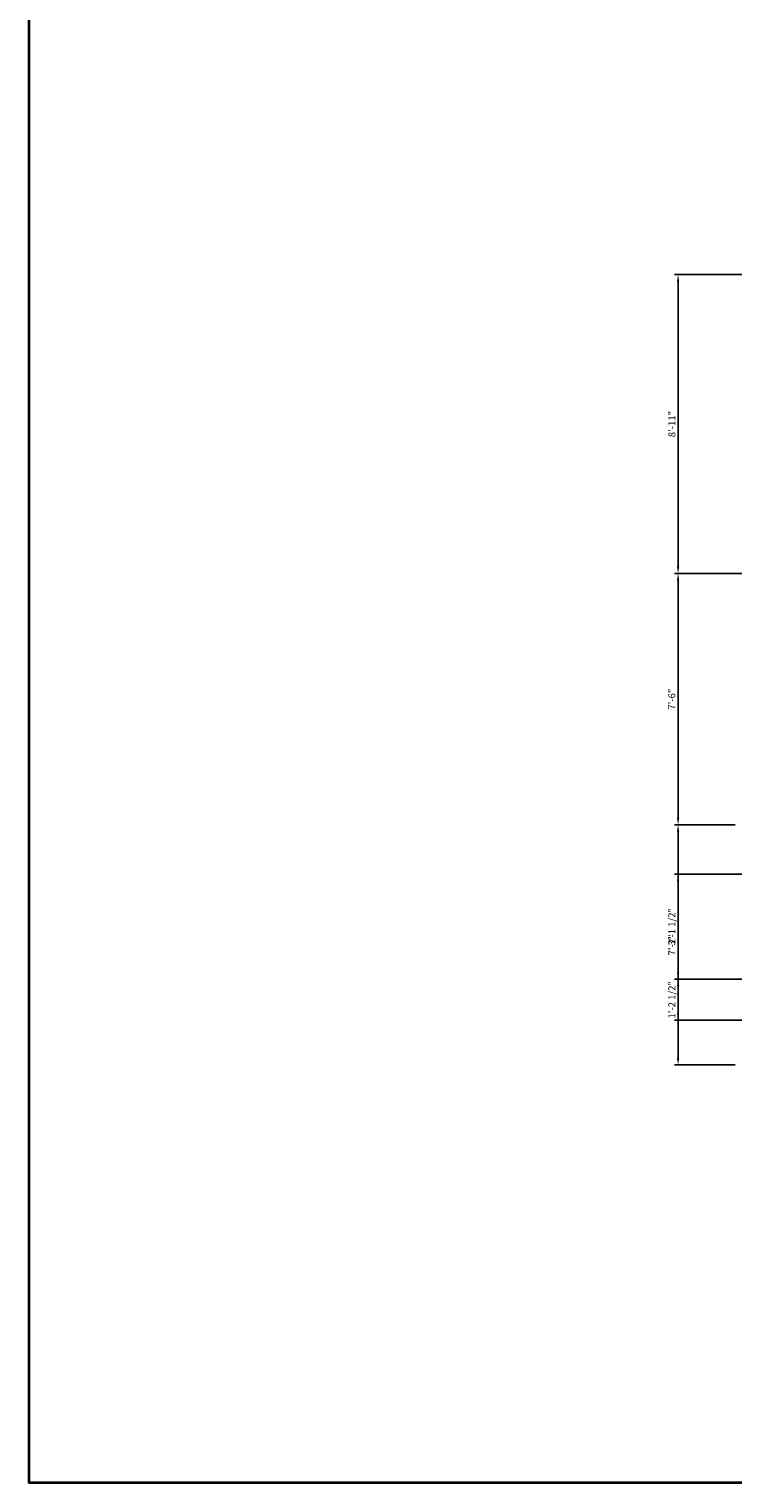
# Model space of a CAD drawing. Units: inches. Extents: x 6038 to 7543, y 3772 to 5131.
# Tile 1 of 14: x 6038 to 6290, y 3772 to 4293. Entities that reach past the tile are written whole.
import ezdxf

# ---------------------------------------------------------------- set-up
doc = ezdxf.new("R2010")
doc.units = ezdxf.units.IN
doc.layers.add('A-ANNO-DIMS', color=4, linetype='Continuous', lineweight=18)
doc.layers.add('A-ANNO-TTLB', color=1, linetype='Continuous', lineweight=35)
doc.styles.get("Standard").update_dxf_attribs({"font": 'arial.ttf'})
doc.dimstyles.new('ISO-25', dxfattribs={"dimtxt": 2.5, "dimasz": 2.5, "dimexe": 1.25, "dimexo": 0.625, "dimtad": 1, "dimdec": 0, "dimlunit": 3, "dimtxsty": 'Standard', "dimcen": 2.5, "dimadec": 0, "dimazin": 0, "dimtfac": 1, "dimtdec": 0, "dimtmove": 0, "dimatfit": 3, "dimfxl": 1, "dimarcsym": 0})

# ---------------------------------------------------------------- blocks, each defined once
blk = doc.blocks.new('*D74')
at = {"layer": 'A-ANNO-DIMS', "color": 0, "lineweight": -2, "transparency": 16777216}
for p, q in [((6290.79, 4007.75), (6269.11, 4007.75)), ((6270.36, 3924.25), (6270.36, 4005.25)), ((6290.79, 3921.75), (6269.11, 3921.75))]:
    blk.add_line(p, q, dxfattribs=at)
at = {"layer": 'A-ANNO-DIMS', "color": 0, "transparency": 16777216}
for points in [[(6269.94, 4005.25), (6270.77, 4005.25), (6270.36, 4007.75)], [(6269.94, 3924.25), (6270.77, 3924.25), (6270.36, 3921.75)]]:
    blk.add_solid(points, dxfattribs=at)
at = {"layer": 'Defpoints', "color": 0, "transparency": 16777216}
for p in [(6270.36, 4007.75), (6291.42, 4007.75), (6291.42, 3921.75)]:
    blk.add_point(p, dxfattribs=at)
at = {"layer": 'A-ANNO-DIMS', "color": 0, "transparency": 16777216, "insert": (6268.48, 3964.75), "char_height": 2.5, "attachment_point": 5, "rotation": 90}
blk.add_mtext('7\'-2"', dxfattribs=at)
blk = doc.blocks.new('*D75')
at = {"layer": 'A-ANNO-DIMS', "color": 0, "lineweight": -2, "transparency": 16777216}
for p, q in [((6308.79, 4097.75), (6269.11, 4097.75)), ((6270.36, 4010.25), (6270.36, 4095.25)), ((6290.79, 4007.75), (6269.11, 4007.75))]:
    blk.add_line(p, q, dxfattribs=at)
at = {"layer": 'A-ANNO-DIMS', "color": 0, "transparency": 16777216}
for points in [[(6269.94, 4095.25), (6270.77, 4095.25), (6270.36, 4097.75)], [(6269.94, 4010.25), (6270.77, 4010.25), (6270.36, 4007.75)]]:
    blk.add_solid(points, dxfattribs=at)
at = {"layer": 'Defpoints', "color": 0, "transparency": 16777216}
for p in [(6270.36, 4097.75), (6309.42, 4097.75), (6291.42, 4007.75)]:
    blk.add_point(p, dxfattribs=at)
at = {"layer": 'A-ANNO-DIMS', "color": 0, "transparency": 16777216, "insert": (6268.46, 4052.75), "char_height": 2.5, "attachment_point": 5, "rotation": 90}
blk.add_mtext('7\'-6"', dxfattribs=at)
blk = doc.blocks.new('*D76')
at = {"layer": 'A-ANNO-DIMS', "color": 0, "lineweight": -2, "transparency": 16777216}
for p, q in [((6308.79, 4204.75), (6269.11, 4204.75)), ((6270.36, 4100.25), (6270.36, 4202.25)), ((6308.79, 4097.75), (6269.11, 4097.75))]:
    blk.add_line(p, q, dxfattribs=at)
at = {"layer": 'A-ANNO-DIMS', "color": 0, "transparency": 16777216}
for points in [[(6269.94, 4202.25), (6270.77, 4202.25), (6270.36, 4204.75)], [(6269.94, 4100.25), (6270.77, 4100.25), (6270.36, 4097.75)]]:
    blk.add_solid(points, dxfattribs=at)
at = {"layer": 'Defpoints', "color": 0, "transparency": 16777216}
for p in [(6270.36, 4204.75), (6309.42, 4204.75), (6309.42, 4097.75)]:
    blk.add_point(p, dxfattribs=at)
at = {"layer": 'A-ANNO-DIMS', "color": 0, "transparency": 16777216, "insert": (6268.46, 4151.25), "char_height": 2.5, "attachment_point": 5, "rotation": 90}
blk.add_mtext('8\'-11"', dxfattribs=at)
blk = doc.blocks.new('*D83')
at = {"layer": 'A-ANNO-DIMS', "color": 0, "lineweight": -2, "transparency": 16777216}
for p, q in [((6448.79, 3952.46), (6269.11, 3952.46)), ((6270.36, 3940.25), (6270.36, 3949.96)), ((6448.79, 3937.75), (6269.11, 3937.75))]:
    blk.add_line(p, q, dxfattribs=at)
at = {"layer": 'A-ANNO-DIMS', "color": 0, "transparency": 16777216}
for points in [[(6269.94, 3949.96), (6270.77, 3949.96), (6270.36, 3952.46)], [(6269.94, 3940.25), (6270.77, 3940.25), (6270.36, 3937.75)]]:
    blk.add_solid(points, dxfattribs=at)
at = {"layer": 'Defpoints', "color": 0, "transparency": 16777216}
for p in [(6270.36, 3952.46), (6449.42, 3952.46), (6449.42, 3937.75)]:
    blk.add_point(p, dxfattribs=at)
at = {"layer": 'A-ANNO-DIMS', "color": 0, "transparency": 16777216, "insert": (6268.44, 3945.1), "char_height": 2.5, "attachment_point": 5, "rotation": 90}
blk.add_mtext('1\'-2 1/2"', dxfattribs=at)
blk = doc.blocks.new('*D84')
at = {"layer": 'A-ANNO-DIMS', "color": 0, "lineweight": -2, "transparency": 16777216}
for p, q in [((6448.79, 3990.02), (6269.11, 3990.02)), ((6270.36, 3954.96), (6270.36, 3987.52)), ((6448.79, 3952.46), (6269.11, 3952.46))]:
    blk.add_line(p, q, dxfattribs=at)
at = {"layer": 'A-ANNO-DIMS', "color": 0, "transparency": 16777216}
for points in [[(6269.94, 3987.52), (6270.77, 3987.52), (6270.36, 3990.02)], [(6269.94, 3954.96), (6270.77, 3954.96), (6270.36, 3952.46)]]:
    blk.add_solid(points, dxfattribs=at)
at = {"layer": 'Defpoints', "color": 0, "transparency": 16777216}
for p in [(6270.36, 3990.02), (6449.42, 3990.02), (6449.42, 3952.46)]:
    blk.add_point(p, dxfattribs=at)
at = {"layer": 'A-ANNO-DIMS', "color": 0, "transparency": 16777216, "insert": (6268.44, 3971.24), "char_height": 2.5, "attachment_point": 5, "rotation": 90}
blk.add_mtext('3\'-1 1/2"', dxfattribs=at)

msp = doc.modelspace()

# ---------------------------------------------------------------- linework, layer by layer
at = {"layer": 'A-ANNO-TTLB'}
msp.add_lwpolyline([(6037.83, 5130.86), (7542.53, 5130.86), (7542.53, 3772.09), (6037.83, 3772.09)], close=True, dxfattribs=at)

# ---------------------------------------------------------------- dimensions: what is measured, and where the dimension line sits
at = {"layer": 'A-ANNO-DIMS'}
for base, p1, p2, picture, middle in [((6270.36, 4204.75), (6309.42, 4097.75), (6309.42, 4204.75), '*D76', (6268.46, 4151.25)), ((6270.36, 4097.75), (6291.42, 4007.75), (6309.42, 4097.75), '*D75', (6268.46, 4052.75)), ((6270.36, 4007.75), (6291.42, 3921.75), (6291.42, 4007.75), '*D74', (6268.48, 3964.75)), ((6270.36, 3990.02), (6449.42, 3952.46), (6449.42, 3990.02), '*D84', (6268.44, 3971.24)), ((6270.36, 3952.46), (6449.42, 3937.75), (6449.42, 3952.46), '*D83', (6268.44, 3945.1))]:
    dim = msp.add_linear_dim(base=base, p1=p1, p2=p2, angle=90, dimstyle='ISO-25', override={"dimdec": 1, "dimlfac": 1, "dimrnd": 0, "dimzin": 1, "dimdsep": 46, "dimlunit": 4, "dimfrac": 2}, dxfattribs=at)
    dim.commit()
    dim.dimension.update_dxf_attribs({"geometry": picture, "text_midpoint": middle})

doc.saveas('drawing.dxf')
